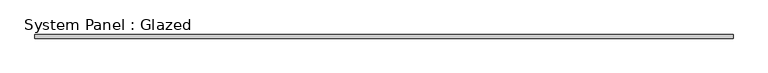
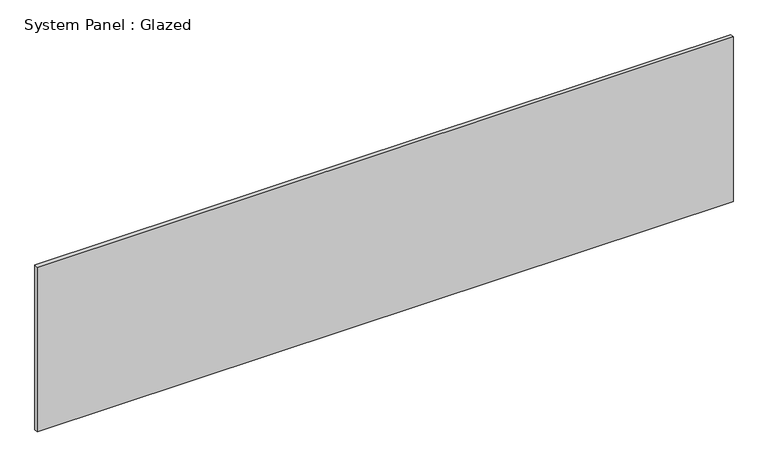
"""IFC4 building model written with IfcOpenShell, lengths in millimetres: plate geometry, System Panel : Glazed."""

from ifc_helpers import new_model, si_unit, origin, origin_with_axes, place, context, project, spatial, polyline, outline, extrude, source, transform, mapped, element, save


def system_panel_glazed_53c2349a(model_context):
    return source(origin(), model_context, "Body", "SweptSolid", [
        extrude(outline(polyline([(2438.4, 19.05), (-2438.4, 19.05), (-2438.4, 44.45), (2438.4, 44.45), (2438.4, 19.05)])), origin_with_axes(), (0.0, 0.0, 1.0), 1219.2),
    ])


if __name__ == "__main__":
    model = new_model("IFC4")
    model_context = context("Model", 3, world=origin())
    ifc_project = project(units=[si_unit("LENGTHUNIT", "METRE", prefix="MILLI")], contexts=[model_context])
    site = spatial("IfcSite", under=ifc_project)
    building = spatial("IfcBuilding", under=site)
    placement = place(None, origin())
    system_panel_glazed_shape = system_panel_glazed_53c2349a(model_context)
    element("IfcPlate", 1, ObjectType="System Panel : Glazed", at=placement, inside=building, context=model_context, shape_type="MappedRepresentation", body=[
        mapped(system_panel_glazed_shape, transform((0.0, 0.0, 0.0), x_axis=(1.0, 0.0, 0.0), y_axis=(0.0, 1.0, 0.0), z_axis=(0.0, 0.0, 1.0))),
    ])
    save(model, "model.ifc")

# Revit data of these elements
# Type "System Panel : Glazed"
#   Construction Type Id = "GSP4R"
#   Analytic Construction = "1/8 in Pilkington single glazing"
#   Visual Light Transmittance = 0.9
#   Solar Heat Gain Coefficient = 0.86
#   Heat Transfer Coefficient (U) = 1.18115 BTU/(h·ft²·°F)
# Element 1 (IfcPlate, "System Panel : Glazed")
#   Materials on its faces: "Glass"
# Materials
#   "Glass": class "Glass", colour RGB 0 128 192, transparency 0.75, Description = "Soda Lime Glass", Cost = 0
